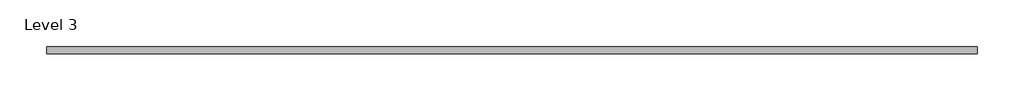
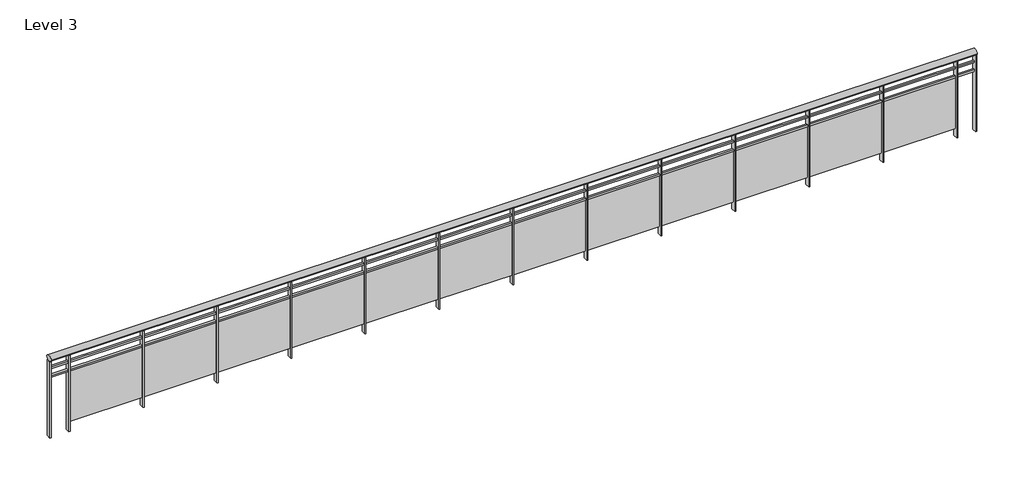
# One storey: 1 railing.
"""IFC4 building model written with IfcOpenShell, lengths in millimetres."""

from ifc_helpers import new_model, si_unit, point, frame, origin, place, context, project, spatial, polyline, ellipse_curve, trimmed, outline, extrude, element, save
from ifc_brep_helpers import plane_surface, extruded_surface, advanced_brep

model = new_model("IFC4")

# Units and contexts
model_context = context("Model", 3, world=origin())
ifc_project = project(units=[si_unit("LENGTHUNIT", "METRE", prefix="MILLI")], contexts=[model_context])

# Site, building, storey
site = spatial("IfcSite", under=ifc_project)
building = spatial("IfcBuilding", under=site)
storey = spatial("IfcBuildingStorey", under=building, Name="Level 3", Elevation=9144.0)

# Railing
placement = place(None, origin())
element("IfcRailing", 1, ObjectType="Glass Panel - Bottom Fill", at=placement, inside=storey, context=model_context, shape_type="SolidModel", body=[
    advanced_brep(
    [(-7102.969584, -549.7943903, 10087.5918347), (-7102.969584, -629.7943903, 10087.5918347), (2911.6217382, -549.7943903, 10087.5918347), (2911.6217382, -629.7943903, 10087.5918347)],
    [
        (0, 1, ellipse_curve(frame((-7102.969584, -589.7943903, 10087.5918347), z_axis=(-1.0, 0.0, 0.0), x_axis=(0.0, -1.0, 0.0)), 40.0, 30.0)),
        (1, 0, ellipse_curve(frame((-7102.969584, -589.7943903, 10087.5918347), z_axis=(-1.0, 0.0, 0.0), x_axis=(0.0, -1.0, 0.0)), 40.0, 30.0)),
        (2, 3, ellipse_curve(frame((2911.6217382, -589.7943903, 10087.5918347), z_axis=(1.0, 0.0, 0.0), x_axis=(0.0, -1.0, 0.0)), 40.0, 30.0)),
        (3, 2, ellipse_curve(frame((2911.6217382, -589.7943903, 10087.5918347), z_axis=(1.0, 0.0, 0.0), x_axis=(0.0, -1.0, 0.0)), 40.0, 30.0)),
        (1, 3),
        (2, 0),
    ],
    [
        plane_surface(frame((-7102.969584, -589.7943903, 10087.5918347), z_axis=(-1.0, 0.0, 0.0), x_axis=(0.0, 1.0, 0.0))),
        plane_surface(frame((2911.6217382, -589.7943903, 10087.5918347), z_axis=(1.0, 0.0, 0.0), x_axis=(0.0, 1.0, 0.0))),
        extruded_surface(trimmed(ellipse_curve(frame((2911.6217382, -589.7943903, 10087.5918347), z_axis=(-1.0, 0.0, 0.0), x_axis=(0.0, -1.0, 0.0)), 40.0, 30.0), [point((2911.6217382, -629.7943903, 10087.5918347))], [point((2911.6217382, -549.7943903, 10087.5918347))], True, "CARTESIAN"), (-10014.5913222, 0.0, 0.0), 10014.5913222),
        extruded_surface(trimmed(ellipse_curve(frame((2911.6217382, -589.7943903, 10087.5918347), z_axis=(-1.0, 0.0, 0.0), x_axis=(0.0, -1.0, 0.0)), 40.0, 30.0), [point((2911.6217382, -549.7943903, 10087.5918347))], [point((2911.6217382, -629.7943903, 10087.5918347))], True, "CARTESIAN"), (-10014.5913222, 0.0, 0.0), 10014.5913222),
    ],
    [
        (0, [[1, 2]]),
        (1, [[3, 4]]),
        (2, [[-2, 5, -3, 6]]),
        (3, [[-1, -6, -4, -5]]),
    ],
),
    extrude(outline(polyline([(-7102.969584, -599.1851555), (-7102.969584, -579.1851555), (2911.6217382, -579.1851555), (2911.6217382, -599.1851555), (-7102.969584, -599.1851555)])), frame((0.0, 0.0, 9967.5918347), z_axis=(0.0, 0.0, 1.0), x_axis=(1.0, 0.0, 0.0)), (0.0, 0.0, 1.0), 20.0),
    extrude(outline(polyline([(-7102.969584, -599.1851555), (-7102.969584, -579.1851555), (2911.6217382, -579.1851555), (2911.6217382, -599.1851555), (-7102.969584, -599.1851555)])), frame((0.0, 0.0, 9867.5918347), z_axis=(0.0, 0.0, 1.0), x_axis=(1.0, 0.0, 0.0)), (0.0, 0.0, 1.0), 20.0),
    extrude(outline(polyline([(2698.3260771, -564.1851555), (2710.3260771, -564.1851555), (2710.3260771, -614.1851555), (2698.3260771, -614.1851555), (2698.3260771, -564.1851555)])), frame((0.0, 0.0, 9187.5918347), z_axis=(0.0, 0.0, 1.0), x_axis=(1.0, 0.0, 0.0)), (0.0, 0.0, 1.0), 869.8465326),
    extrude(outline(polyline([(1904.3260771, -590.9099656), (2704.3260771, -590.9099656), (2704.3260771, -595.9099656), (1904.3260771, -595.9099656), (1904.3260771, -590.9099656)])), frame((0.0, 0.0, 9287.5918347), z_axis=(0.0, 0.0, 1.0), x_axis=(1.0, 0.0, 0.0)), (0.0, 0.0, 1.0), 580.0),
    extrude(outline(polyline([(1898.3260771, -564.1851555), (1910.3260771, -564.1851555), (1910.3260771, -614.1851555), (1898.3260771, -614.1851555), (1898.3260771, -564.1851555)])), frame((0.0, 0.0, 9187.5918347), z_axis=(0.0, 0.0, 1.0), x_axis=(1.0, 0.0, 0.0)), (0.0, 0.0, 1.0), 869.8465326),
    extrude(outline(polyline([(1104.3260771, -590.9099656), (1904.3260771, -590.9099656), (1904.3260771, -595.9099656), (1104.3260771, -595.9099656), (1104.3260771, -590.9099656)])), frame((0.0, 0.0, 9287.5918347), z_axis=(0.0, 0.0, 1.0), x_axis=(1.0, 0.0, 0.0)), (0.0, 0.0, 1.0), 580.0),
    extrude(outline(polyline([(1098.3260771, -564.1851555), (1110.3260771, -564.1851555), (1110.3260771, -614.1851555), (1098.3260771, -614.1851555), (1098.3260771, -564.1851555)])), frame((0.0, 0.0, 9187.5918347), z_axis=(0.0, 0.0, 1.0), x_axis=(1.0, 0.0, 0.0)), (0.0, 0.0, 1.0), 869.8465326),
    extrude(outline(polyline([(304.3260771, -590.9099656), (1104.3260771, -590.9099656), (1104.3260771, -595.9099656), (304.3260771, -595.9099656), (304.3260771, -590.9099656)])), frame((0.0, 0.0, 9287.5918347), z_axis=(0.0, 0.0, 1.0), x_axis=(1.0, 0.0, 0.0)), (0.0, 0.0, 1.0), 580.0),
    extrude(outline(polyline([(298.3260771, -564.1851555), (310.3260771, -564.1851555), (310.3260771, -614.1851555), (298.3260771, -614.1851555), (298.3260771, -564.1851555)])), frame((0.0, 0.0, 9187.5918347), z_axis=(0.0, 0.0, 1.0), x_axis=(1.0, 0.0, 0.0)), (0.0, 0.0, 1.0), 869.8465326),
    extrude(outline(polyline([(-495.6739229, -590.9099656), (304.3260771, -590.9099656), (304.3260771, -595.9099656), (-495.6739229, -595.9099656), (-495.6739229, -590.9099656)])), frame((0.0, 0.0, 9287.5918347), z_axis=(0.0, 0.0, 1.0), x_axis=(1.0, 0.0, 0.0)), (0.0, 0.0, 1.0), 580.0),
    extrude(outline(polyline([(-501.6739229, -564.1851555), (-489.6739229, -564.1851555), (-489.6739229, -614.1851555), (-501.6739229, -614.1851555), (-501.6739229, -564.1851555)])), frame((0.0, 0.0, 9187.5918347), z_axis=(0.0, 0.0, 1.0), x_axis=(1.0, 0.0, 0.0)), (0.0, 0.0, 1.0), 869.8465326),
    extrude(outline(polyline([(-1295.6739229, -590.9099656), (-495.6739229, -590.9099656), (-495.6739229, -595.9099656), (-1295.6739229, -595.9099656), (-1295.6739229, -590.9099656)])), frame((0.0, 0.0, 9287.5918347), z_axis=(0.0, 0.0, 1.0), x_axis=(1.0, 0.0, 0.0)), (0.0, 0.0, 1.0), 580.0),
    extrude(outline(polyline([(-1301.6739229, -564.1851555), (-1289.6739229, -564.1851555), (-1289.6739229, -614.1851555), (-1301.6739229, -614.1851555), (-1301.6739229, -564.1851555)])), frame((0.0, 0.0, 9187.5918347), z_axis=(0.0, 0.0, 1.0), x_axis=(1.0, 0.0, 0.0)), (0.0, 0.0, 1.0), 869.8465326),
    extrude(outline(polyline([(-2095.6739229, -590.9099656), (-1295.6739229, -590.9099656), (-1295.6739229, -595.9099656), (-2095.6739229, -595.9099656), (-2095.6739229, -590.9099656)])), frame((0.0, 0.0, 9287.5918347), z_axis=(0.0, 0.0, 1.0), x_axis=(1.0, 0.0, 0.0)), (0.0, 0.0, 1.0), 580.0),
    extrude(outline(polyline([(-2101.6739229, -564.1851555), (-2089.6739229, -564.1851555), (-2089.6739229, -614.1851555), (-2101.6739229, -614.1851555), (-2101.6739229, -564.1851555)])), frame((0.0, 0.0, 9187.5918347), z_axis=(0.0, 0.0, 1.0), x_axis=(1.0, 0.0, 0.0)), (0.0, 0.0, 1.0), 869.8465326),
    extrude(outline(polyline([(-2895.6739229, -590.9099656), (-2095.6739229, -590.9099656), (-2095.6739229, -595.9099656), (-2895.6739229, -595.9099656), (-2895.6739229, -590.9099656)])), frame((0.0, 0.0, 9287.5918347), z_axis=(0.0, 0.0, 1.0), x_axis=(1.0, 0.0, 0.0)), (0.0, 0.0, 1.0), 580.0),
    extrude(outline(polyline([(-2901.6739229, -564.1851555), (-2889.6739229, -564.1851555), (-2889.6739229, -614.1851555), (-2901.6739229, -614.1851555), (-2901.6739229, -564.1851555)])), frame((0.0, 0.0, 9187.5918347), z_axis=(0.0, 0.0, 1.0), x_axis=(1.0, 0.0, 0.0)), (0.0, 0.0, 1.0), 869.8465326),
    extrude(outline(polyline([(-3695.6739229, -590.9099656), (-2895.6739229, -590.9099656), (-2895.6739229, -595.9099656), (-3695.6739229, -595.9099656), (-3695.6739229, -590.9099656)])), frame((0.0, 0.0, 9287.5918347), z_axis=(0.0, 0.0, 1.0), x_axis=(1.0, 0.0, 0.0)), (0.0, 0.0, 1.0), 580.0),
    extrude(outline(polyline([(-3701.6739229, -564.1851555), (-3689.6739229, -564.1851555), (-3689.6739229, -614.1851555), (-3701.6739229, -614.1851555), (-3701.6739229, -564.1851555)])), frame((0.0, 0.0, 9187.5918347), z_axis=(0.0, 0.0, 1.0), x_axis=(1.0, 0.0, 0.0)), (0.0, 0.0, 1.0), 869.8465326),
    extrude(outline(polyline([(-4495.6739229, -590.9099656), (-3695.6739229, -590.9099656), (-3695.6739229, -595.9099656), (-4495.6739229, -595.9099656), (-4495.6739229, -590.9099656)])), frame((0.0, 0.0, 9287.5918347), z_axis=(0.0, 0.0, 1.0), x_axis=(1.0, 0.0, 0.0)), (0.0, 0.0, 1.0), 580.0),
    extrude(outline(polyline([(-4501.6739229, -564.1851555), (-4489.6739229, -564.1851555), (-4489.6739229, -614.1851555), (-4501.6739229, -614.1851555), (-4501.6739229, -564.1851555)])), frame((0.0, 0.0, 9187.5918347), z_axis=(0.0, 0.0, 1.0), x_axis=(1.0, 0.0, 0.0)), (0.0, 0.0, 1.0), 869.8465326),
    extrude(outline(polyline([(-5295.6739229, -590.9099656), (-4495.6739229, -590.9099656), (-4495.6739229, -595.9099656), (-5295.6739229, -595.9099656), (-5295.6739229, -590.9099656)])), frame((0.0, 0.0, 9287.5918347), z_axis=(0.0, 0.0, 1.0), x_axis=(1.0, 0.0, 0.0)), (0.0, 0.0, 1.0), 580.0),
    extrude(outline(polyline([(-5301.6739229, -564.1851555), (-5289.6739229, -564.1851555), (-5289.6739229, -614.1851555), (-5301.6739229, -614.1851555), (-5301.6739229, -564.1851555)])), frame((0.0, 0.0, 9187.5918347), z_axis=(0.0, 0.0, 1.0), x_axis=(1.0, 0.0, 0.0)), (0.0, 0.0, 1.0), 869.8465326),
    extrude(outline(polyline([(-6095.6739229, -590.9099656), (-5295.6739229, -590.9099656), (-5295.6739229, -595.9099656), (-6095.6739229, -595.9099656), (-6095.6739229, -590.9099656)])), frame((0.0, 0.0, 9287.5918347), z_axis=(0.0, 0.0, 1.0), x_axis=(1.0, 0.0, 0.0)), (0.0, 0.0, 1.0), 580.0),
    extrude(outline(polyline([(-6101.6739229, -564.1851555), (-6089.6739229, -564.1851555), (-6089.6739229, -614.1851555), (-6101.6739229, -614.1851555), (-6101.6739229, -564.1851555)])), frame((0.0, 0.0, 9187.5918347), z_axis=(0.0, 0.0, 1.0), x_axis=(1.0, 0.0, 0.0)), (0.0, 0.0, 1.0), 869.8465326),
    extrude(outline(polyline([(-6895.6739229, -590.9099656), (-6095.6739229, -590.9099656), (-6095.6739229, -595.9099656), (-6895.6739229, -595.9099656), (-6895.6739229, -590.9099656)])), frame((0.0, 0.0, 9287.5918347), z_axis=(0.0, 0.0, 1.0), x_axis=(1.0, 0.0, 0.0)), (0.0, 0.0, 1.0), 580.0),
    extrude(outline(polyline([(-6901.6739229, -564.1851555), (-6889.6739229, -564.1851555), (-6889.6739229, -614.1851555), (-6901.6739229, -614.1851555), (-6901.6739229, -564.1851555)])), frame((0.0, 0.0, 9187.5918347), z_axis=(0.0, 0.0, 1.0), x_axis=(1.0, 0.0, 0.0)), (0.0, 0.0, 1.0), 869.8465326),
    extrude(outline(polyline([(2903.6217382, -564.1851555), (2915.6217382, -564.1851555), (2915.6217382, -614.1851555), (2903.6217382, -614.1851555), (2903.6217382, -564.1851555)])), frame((0.0, 0.0, 9187.5918347), z_axis=(0.0, 0.0, 1.0), x_axis=(1.0, 0.0, 0.0)), (0.0, 0.0, 1.0), 869.8465326),
    extrude(outline(polyline([(-7106.969584, -564.1851555), (-7094.969584, -564.1851555), (-7094.969584, -614.1851555), (-7106.969584, -614.1851555), (-7106.969584, -564.1851555)])), frame((0.0, 0.0, 9187.5918347), z_axis=(0.0, 0.0, 1.0), x_axis=(1.0, 0.0, 0.0)), (0.0, 0.0, 1.0), 869.8465326),
])

save(model, "model.ifc")

# Revit data of these elements
# Type "Glass Panel - Bottom Fill"
#   built-in parameter 1008612 = 0.019685 (stored number, unit not read)
#   built-in parameter 1008611 = 0.019685 (stored number, unit not read)
#   built-in parameter 1008609 = 0.902231 (stored number, unit not read)
#   built-in parameter 1008604 = 0.19685 (stored number, unit not read)
#   built-in parameter 1008603 = 0.164042 (stored number, unit not read)
#   Railing Height = 2' - 11.43307"
#   built-in parameter 1008630 = 2
#   built-in parameter 1008610 = 2
# Element 1 (IfcRailing, "Glass Panel - Bottom Fill")
#   built-in parameter 1008621 = 0.143018 (stored number, unit not read)
#   Phase Created = New Construction
#   Materials on its faces: "Metal - Stainless Steel,Polished", "Glass"
# Materials
#   "Metal - Stainless Steel,Polished": class "Metal", colour RGB 189 187 185, transparency 0, Cost = 0
#   "Glass": class "Glass", colour RGB 218 227 224, transparency 0.85, Description = "Soda Lime Glass", Cost = 0
